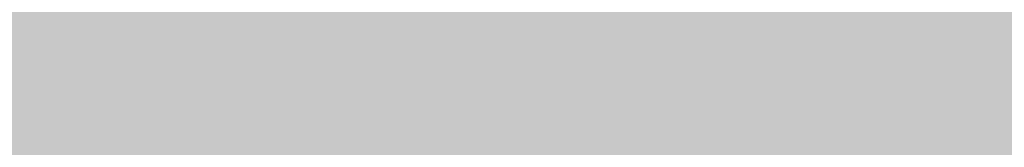
# Model space of a CAD drawing. Units: inches. Extents: x 2083 to 3317, y 1141 to 2115.
# Tile 68 of 256: x 2238.294 to 2242.452, y 1477.116 to 1477.656. Entities that reach past the tile are written whole.
import ezdxf

# ---------------------------------------------------------------- set-up
doc = ezdxf.new("R2010")
doc.units = ezdxf.units.IN
doc.layers.add('A-ANNO-DIMS', color=2, linetype='Continuous', lineweight=18)
doc.layers.add('A-WALL-PATT', color=251, linetype='Continuous', lineweight=13, true_color=0x636466)
doc.styles.get("Standard").update_dxf_attribs({"font": 'arial.ttf'})
doc.dimstyles.new('ISO-25', dxfattribs={"dimtxt": 12, "dimasz": 12, "dimexe": 1.25, "dimexo": 0.625, "dimtad": 1, "dimlunit": 3, "dimtxsty": 'Standard', "dimcen": 2.5, "dimadec": 0, "dimazin": 0, "dimtfac": 1, "dimtmove": 0, "dimatfit": 3, "dimfxl": 1, "dimarcsym": 0})

# ---------------------------------------------------------------- blocks, each defined once
blk = doc.blocks.new('*D30')
at = {"layer": 'A-ANNO-DIMS', "color": 0, "lineweight": -2, "transparency": 16777216}
for p, q in [((2240.0179, 1445.2738), (2240.0179, 1448.0455)), ((2254.3293, 1445.2738), (2254.3293, 1448.0455)), ((2228.0179, 1446.7955), (2216.0179, 1446.7955)), ((2240.0179, 1446.7955), (2254.3293, 1446.7955)), ((2266.3293, 1446.7955), (2413.7649, 1446.7955))]:
    blk.add_line(p, q, dxfattribs=at)
at = {"layer": 'A-ANNO-DIMS', "color": 0, "transparency": 16777216}
for points in [[(2228.0179, 1448.7955), (2228.0179, 1444.7955), (2240.0179, 1446.7955)], [(2266.3293, 1448.7955), (2266.3293, 1444.7955), (2254.3293, 1446.7955)]]:
    blk.add_solid(points, dxfattribs=at)
at = {"layer": 'Defpoints', "color": 0, "transparency": 16777216}
for p in [(2254.3293, 1446.7955), (2240.0179, 1444.6488), (2254.3293, 1444.6488)]:
    blk.add_point(p, dxfattribs=at)
at = {"layer": 'A-ANNO-DIMS', "color": 0, "transparency": 16777216, "insert": (2346.0471, 1453.6252), "char_height": 12, "attachment_point": 5}
blk.add_mtext('WC 1\'-2 1/2" TYP.', dxfattribs=at)
blk = doc.blocks.new('*D31')
at = {"layer": 'A-ANNO-DIMS', "color": 0, "lineweight": -2, "transparency": 16777216}
for p, q in [((2237.8711, 1456.6488), (2237.8711, 1541.9152)), ((2239.3929, 1444.6488), (2236.6211, 1444.6488)), ((2237.8711, 1431.5475), (2237.8711, 1444.6488)), ((2239.3929, 1431.5475), (2236.6211, 1431.5475)), ((2237.8711, 1419.5475), (2237.8711, 1407.5475))]:
    blk.add_line(p, q, dxfattribs=at)
at = {"layer": 'A-ANNO-DIMS', "color": 0, "transparency": 16777216}
for points in [[(2235.8711, 1456.6488), (2239.8711, 1456.6488), (2237.8711, 1444.6488)], [(2235.8711, 1419.5475), (2239.8711, 1419.5475), (2237.8711, 1431.5475)]]:
    blk.add_solid(points, dxfattribs=at)
at = {"layer": 'Defpoints', "color": 0, "transparency": 16777216}
for p in [(2237.8711, 1444.6488), (2240.0179, 1444.6488), (2240.0179, 1431.5475)]:
    blk.add_point(p, dxfattribs=at)
at = {"layer": 'A-ANNO-DIMS', "color": 0, "transparency": 16777216, "insert": (2231.2175, 1505.282), "char_height": 12, "attachment_point": 5, "rotation": 90}
blk.add_mtext('1\'-1" TYP.', dxfattribs=at)
blk = doc.blocks.new('*D62')
at = {"layer": 'A-ANNO-DIMS', "color": 0, "lineweight": -2, "transparency": 16777216}
for p, q in [((2235.9598, 1469.3864), (2235.9598, 1522.3614)), ((2379.9598, 1469.3864), (2379.9598, 1522.3614)), ((2247.9598, 1521.1114), (2367.9598, 1521.1114))]:
    blk.add_line(p, q, dxfattribs=at)
at = {"layer": 'A-ANNO-DIMS', "color": 0, "transparency": 16777216}
for points in [[(2247.9598, 1523.1114), (2247.9598, 1519.1114), (2235.9598, 1521.1114)], [(2367.9598, 1523.1114), (2367.9598, 1519.1114), (2379.9598, 1521.1114)]]:
    blk.add_solid(points, dxfattribs=at)
at = {"layer": 'Defpoints', "color": 0, "transparency": 16777216}
for p in [(2379.9598, 1521.1114), (2235.9598, 1468.7614), (2379.9598, 1468.7614)]:
    blk.add_point(p, dxfattribs=at)
at = {"layer": 'A-ANNO-DIMS', "color": 0, "transparency": 16777216, "insert": (2307.9598, 1527.8632), "char_height": 12, "attachment_point": 5}
blk.add_mtext('12\'-0"', dxfattribs=at)

msp = doc.modelspace()

# ---------------------------------------------------------------- hatches: boundary and pattern name
at = {"layer": 'A-WALL-PATT'}
h = msp.add_hatch(color=256, dxfattribs=at)
h.dxf.hatch_style = 1
h.paths.add_polyline_path([(3126.9598, 2020.7614), (2748.9598, 2020.7614), (2604.9598, 2020.7614), (2226.9598, 2020.7614), (2226.9598, 1702.7614), (2466.9598, 1702.7614), (2466.9598, 1582.7614), (2418.9598, 1582.7614), (2418.9598, 1477.7614), (2226.9598, 1477.7614), (2226.9598, 1263.2614), (2544.9598, 1263.2614), (2544.9598, 1411.7614), (2604.9598, 1411.7614), (2685.9598, 1411.7614), (2685.9598, 1420.7614), (2604.9598, 1420.7614), (2604.9598, 1573.7614), (2604.9598, 1702.7614), (2604.9598, 2011.7614), (2748.9598, 2011.7614), (2748.9598, 1702.7614), (2862.9598, 1702.7614), (2862.9598, 1621.7614), (2871.9598, 1621.7614), (2871.9598, 1702.7614), (2883.9598, 1702.7614), (2883.9598, 1706.9395, -0.026459), (2883.9598, 1711.7614), (2757.9598, 1711.7614), (2757.9598, 1807.7614), (2787.9598, 1807.7614), (2787.9598, 1812.2614), (2757.9598, 1812.2614), (2757.9598, 2011.7614), (2877.9598, 2011.7614), (2877.9598, 1812.2614), (2847.9598, 1812.2614), (2847.9598, 1807.7614), (2889.8357, 1807.7614), (2889.8357, 1812.2614), (2882.4598, 1812.2614), (2882.4598, 2011.7614), (3117.9598, 2011.7614), (3117.9598, 1812.2614), (2937.8357, 1812.2614), (2937.8357, 1807.7614), (2995.7098, 1807.7614), (2995.7098, 1796.1177), (3000.2098, 1796.1177), (3000.2098, 1807.7614), (3117.9598, 1807.7614), (3117.9598, 1711.7614), (3000.2098, 1711.7614), (3000.2098, 1760.1177), (2998.5727, 1760.1177, -0.020711), (2995.7098, 1760.1177), (2995.7098, 1711.7614), (2931.9598, 1711.7614), (2931.9598, 1702.7614), (3126.9598, 1702.7614)])
h.paths.add_polyline_path([(2471.4598, 2011.7614), (2471.4598, 1810.0114), (2462.7169, 1810.0114), (2462.7169, 1805.5114), (2505.9598, 1805.5114), (2505.9598, 1810.0114), (2475.9598, 1810.0114), (2475.9598, 2011.7614), (2595.9598, 2011.7614), (2595.9598, 1810.0114), (2565.9598, 1810.0114), (2565.9598, 1805.5114), (2595.9598, 1805.5114), (2595.9598, 1711.7614), (2235.9598, 1711.7614), (2235.9598, 1805.5114), (2353.7098, 1805.5114), (2353.7098, 1796.0542), (2358.2098, 1796.0542), (2358.2098, 1805.5114), (2414.7169, 1805.5114), (2414.7169, 1810.0114), (2235.9598, 1810.0114), (2235.9598, 2011.7614)], flags=16)
h.paths.add_polyline_path([(2270.2047, 1994.61), (2270.2047, 1970.61), (2246.2047, 1970.61), (2246.2047, 1994.61)], flags=0)
edge = h.paths.add_edge_path(flags=0)
edge.add_ellipse((2332.0274, 1899.7982), major_axis=(-3.043, 3.043), ratio=0.168252, start_angle=-161.3322, end_angle=-156.3071, ccw=False)
edge.add_ellipse((2333.082, 1898.7435), major_axis=(-1.0546, 1.0546), ratio=0.453532, start_angle=-123.371, end_angle=-94.1591)
edge = h.paths.add_edge_path(flags=0)
edge.add_ellipse((2332.0274, 1968.8763), major_axis=(3.043, 3.043), ratio=0.168252, start_angle=18.6678, end_angle=23.6929)
edge.add_spline(control_points=[(2332.9256, 1970.6911), (2332.2268, 1970.3361), (2330.8937, 1969.6589), (2328.4131, 1970.9321), (2327.2039, 1967.7487), (2324.7096, 1969.9556), (2322.5328, 1967.0124), (2320.0128, 1971.2958), (2317.6803, 1968.1578), (2316.0405, 1967.102), (2315.4269, 1966.8096)], knot_values=[0, 0, 0, 0, 2.267059, 4.324559, 6.685584, 8.878641, 11.121502, 14.300359, 17.755284, 19.732645, 19.732645, 19.732645, 19.732645], degree=3, periodic=0)
edge.add_ellipse((2332.0274, 1968.8763), major_axis=(3.043, 3.043), ratio=0.168252, start_angle=18.6678, end_angle=23.6929, ccw=False)
edge.add_ellipse((2333.082, 1969.9309), major_axis=(1.0546, 1.0546), ratio=0.453532, start_angle=56.629, end_angle=85.8409, ccw=False)
edge = h.paths.add_edge_path(flags=0)
edge.add_spline(control_points=[(2296.4283, 1967.9879), (2293.6278, 1965.3363), (2287.7036, 1959.7271), (2299.7439, 1949.9957), (2294.5326, 1935.6685), (2290.5732, 1920.6035), (2293.3941, 1909.9737), (2296.1854, 1904.9665)], knot_values=[0.099185, 0.099185, 0.099185, 0.099185, 0.345301, 0.619822, 0.982653, 1.386093, 1.810555, 1.810555, 1.810555, 1.810555], degree=3, periodic=0)
edge.add_spline(control_points=[(2296.1854, 1904.9665), (2297.3836, 1902.6193), (2298.001, 1901.9493), (2298.553, 1901.4682)], knot_values=[0.006246, 0.006246, 0.006246, 0.006246, 0.055476, 0.055476, 0.055476, 0.055476], degree=3, periodic=0)
edge.add_spline(control_points=[(2298.553, 1901.4682), (2297.2586, 1900.9232), (2295.2253, 1900.2321), (2293.0602, 1900.6142), (2292.1014, 1900.7884), (2292.0896, 1900.7906)], knot_values=[0.312835, 0.312835, 0.312835, 0.312835, 0.40178, 0.474987, 0.475903, 0.475903, 0.475903, 0.475903], degree=3, periodic=0)
edge.add_arc((2292.7936, 1904.6641), 3.937, 215.4209, 259.6982, ccw=False)
edge.add_spline(control_points=[(2289.5853, 1902.3823), (2289.4767, 1902.5351), (2289.3685, 1902.688), (2289.2609, 1902.8412)], knot_values=[0.102872, 0.102872, 0.102872, 0.102872, 0.116896, 0.116896, 0.116896, 0.116896], degree=3, periodic=0)
edge.add_spline(control_points=[(2289.2609, 1902.8412), (2288.6866, 1902.5502), (2287.64, 1902.0199), (2285.8813, 1901.874), (2283.853, 1901.5044), (2281.72, 1899.7105), (2278.467, 1899.4929), (2276.1571, 1901.8832), (2272.259, 1899.8041), (2267.7776, 1901.8432), (2262.2439, 1900.184), (2257.4149, 1901.7821), (2254.3184, 1900.7261), (2253.1783, 1900.3373)], knot_values=[0, 0, 0, 0, 1.907977, 3.477176, 5.261074, 7.972851, 11.680248, 13.717921, 16.939592, 22.789562, 27.502503, 33.595215, 37.145618, 37.145618, 37.145618, 37.145618], degree=3, periodic=0)
edge.add_line((2253.1783, 1900.3373), (2250.2442, 1902.8412))
edge.add_line((2250.2442, 1902.8412), (2250.2442, 1965.8333))
edge.add_line((2250.2442, 1965.8333), (2253.1783, 1968.3371))
edge.add_spline(control_points=[(2253.1783, 1968.3371), (2254.3184, 1967.9483), (2257.4149, 1966.8924), (2262.2439, 1968.4904), (2267.7776, 1966.8313), (2271.5267, 1968.5372), (2273.8759, 1967.8283), (2274.2067, 1967.7276)], knot_values=[0, 0, 0, 0, 0.09018, 0.244935, 0.364644, 0.513233, 0.537855, 0.537855, 0.537855, 0.537855], degree=3, periodic=0)
edge.add_arc((2274.3529, 1963.7933), 3.937, 72.0511, 92.1279, ccw=False)
edge.add_arc((2281.2969, 1985.23), 18.5963, 252.05113, 288.56572)
edge.add_arc((2292.3167, 1956.0289), 12.6461, 71.02679, 113.77822, ccw=False)
edge = h.paths.add_edge_path(flags=0)
edge.add_spline(control_points=[(2274.8994, 1951.8562), (2275.0662, 1951.6166), (2275.2327, 1951.3766), (2275.398, 1951.1359)], knot_values=[1.409916, 1.409916, 1.409916, 1.409916, 1.43159, 1.43159, 1.43159, 1.43159], degree=3, periodic=0)
edge.add_spline(control_points=[(2275.398, 1951.1359), (2275.7921, 1950.5619), (2276.1792, 1949.9838), (2276.5455, 1949.3971)], knot_values=[1.358238, 1.358238, 1.358238, 1.358238, 1.409916, 1.409916, 1.409916, 1.409916], degree=3, periodic=0)
edge.add_line((2276.5455, 1949.3971), (2277.4373, 1947.8622))
edge.add_spline(control_points=[(2277.4373, 1947.8622), (2276.3038, 1945.6731), (2274.6397, 1942.4269), (2274.6316, 1938.0939), (2272.7991, 1930.8515), (2274.3564, 1943.897), (2275.9477, 1947.9234), (2276.5455, 1949.3971)], knot_values=[0.005632, 0.005632, 0.005632, 0.005632, 0.186014, 0.266002, 0.357087, 0.59639, 0.739732, 0.739732, 0.739732, 0.739732], degree=3, periodic=0)
edge.add_spline(control_points=[(2276.5455, 1949.3971), (2276.1792, 1949.9838), (2275.7921, 1950.5619), (2275.398, 1951.1359)], knot_values=[1.358238, 1.358238, 1.358238, 1.358238, 1.409916, 1.409916, 1.409916, 1.409916], degree=3, periodic=0)
edge.add_spline(control_points=[(2275.398, 1951.1359), (2274.9425, 1950.0805), (2274.2078, 1948.0253), (2273.9346, 1944.8515), (2272.4685, 1937.6275), (2273.4662, 1945.6965), (2274.7006, 1951.0595), (2274.8994, 1951.8562)], knot_values=[0.104364, 0.104364, 0.104364, 0.104364, 0.189636, 0.269624, 0.36071, 0.600013, 0.644622, 0.644622, 0.644622, 0.644622], degree=3, periodic=0)
h.paths.add_polyline_path([(2269.1675, 1963.1276, -0.357527), (2268.1706, 1960.9764, -0.092561), (2268.1706, 1939.4363, -0.357527), (2269.1675, 1937.2851, -0.357527), (2267.0163, 1938.282, -0.164785), (2254.6856, 1938.282, -0.357527), (2252.5344, 1937.2851, -0.357527), (2253.5313, 1939.4363, -0.092561), (2253.5313, 1960.9764, -0.357527), (2252.5344, 1963.1276, -0.357527), (2254.6856, 1962.1307, -0.164785), (2267.0163, 1962.1307, -0.357527)], flags=0)
h.paths.add_polyline_path([(2248.8741, 1967.8018), (2248.8741, 1957.0277), (2249.4578, 1957.0277), (2249.4578, 1911.6468), (2248.8741, 1911.6468), (2248.8741, 1900.8727), (2246.5119, 1900.8727, 0.197327), (2244.1497, 1902.4569), (2244.1497, 1966.2176, 0.197327), (2246.5119, 1967.8018)], flags=0)
h.paths.add_polyline_path([(2269.1675, 1931.3893, -0.357527), (2268.1706, 1929.2381, -0.092561), (2268.1706, 1907.6981, -0.357527), (2269.1675, 1905.5469, -0.357527), (2267.0163, 1906.5438, -0.164785), (2254.6856, 1906.5438, -0.357527), (2252.5344, 1905.5469, -0.357527), (2253.5313, 1907.6981, -0.092561), (2253.5313, 1929.2381, -0.357527), (2252.5344, 1931.3893, -0.357527), (2254.6856, 1930.3925, -0.164785), (2267.0163, 1930.3925, -0.357527)], flags=0)
edge = h.paths.add_edge_path(flags=0)
edge.add_spline(control_points=[(2276.1969, 1906.7237), (2276.1681, 1909.0289), (2276.114, 1913.3719), (2270.5984, 1924.925), (2273.9052, 1919.0128), (2275.9217, 1916.2621), (2275.4746, 1912.4021), (2277.2579, 1910.3806), (2276.696, 1908.225), (2276.6462, 1906.813), (2276.6178, 1906.0084)], knot_values=[0, 0, 0, 0, 8.61026, 16.221274, 18.843057, 23.804898, 27.440828, 29.356102, 31.203478, 33.650687, 33.650687, 33.650687, 33.650687], degree=3, periodic=0)
edge.add_spline(control_points=[(2276.6178, 1906.0084), (2276.6233, 1905.6241), (2276.4977, 1904.6287), (2275.4418, 1903.8547), (2274.9373, 1903.0804), (2274.8591, 1902.8412)], knot_values=[0.156488, 0.156488, 0.156488, 0.156488, 0.184398, 0.231376, 0.250598, 0.250598, 0.250598, 0.250598], degree=3, periodic=0)
edge.add_line((2274.8591, 1902.8412), (2276.506, 1902.8412))
edge.add_spline(control_points=[(2276.506, 1902.8412), (2276.7883, 1903.0849), (2277.6651, 1904.1252), (2278.2495, 1904.3407), (2277.6539, 1908.5274), (2278.1557, 1906.2278), (2278.1005, 1905.2859), (2278.8467, 1904.069), (2277.8568, 1903.4149), (2277.8742, 1902.991), (2277.9036, 1902.8412)], knot_values=[0.059574, 0.059574, 0.059574, 0.059574, 0.080753, 0.103741, 0.16972, 0.176036, 0.207137, 0.240474, 0.262341, 0.27366, 0.27366, 0.27366, 0.27366], degree=3, periodic=0)
edge.add_line((2277.9036, 1902.8412), (2280.0298, 1902.8412))
edge.add_spline(control_points=[(2280.0298, 1902.8412), (2279.8882, 1903.0884), (2279.4993, 1903.9816), (2280.1523, 1905.9393), (2278.1036, 1909.6578), (2279.7624, 1907.1853), (2280.3279, 1904.8749), (2280.4851, 1903.4896), (2281.4633, 1903.2494), (2281.7583, 1902.9365), (2281.834, 1902.8412)], knot_values=[0.013856, 0.013856, 0.013856, 0.013856, 0.034874, 0.088867, 0.107879, 0.126738, 0.158714, 0.193757, 0.217487, 0.226722, 0.226722, 0.226722, 0.226722], degree=3, periodic=0)
edge.add_spline(control_points=[(2281.834, 1902.8412), (2281.7875, 1902.8267), (2281.647, 1902.783), (2281.3955, 1902.8595), (2281.0881, 1902.9852), (2280.7207, 1903.0609), (2280.3335, 1903.0257), (2280.1248, 1902.8989), (2280.0298, 1902.8412)], knot_values=[0, 0, 0, 0, 0.14413, 0.435517, 0.749276, 1.153046, 1.548371, 1.878348, 1.878348, 1.878348, 1.878348], degree=3, periodic=0)
edge.add_line((2280.0298, 1902.8412), (2277.9036, 1902.8412))
edge.add_spline(control_points=[(2277.9036, 1902.8412), (2277.8929, 1902.7959), (2277.8654, 1902.6796), (2277.6075, 1902.6875), (2277.2741, 1902.8007), (2276.8379, 1902.6198), (2276.5838, 1902.7893), (2276.506, 1902.8412)], knot_values=[0, 0, 0, 0, 0.127189, 0.326199, 0.628009, 1.24357, 1.515331, 1.515331, 1.515331, 1.515331], degree=3, periodic=0)
edge.add_line((2276.506, 1902.8412), (2274.8591, 1902.8412))
edge.add_spline(control_points=[(2274.8591, 1902.8412), (2274.8144, 1902.8986), (2274.7251, 1903.0134), (2274.4935, 1903.119), (2274.2443, 1902.9605), (2273.9371, 1903.1849), (2273.614, 1902.9831), (2273.4083, 1902.883), (2273.3223, 1902.8412)], knot_values=[0, 0, 0, 0, 0.21843, 0.436957, 0.687977, 0.990379, 1.398396, 1.69185, 1.69185, 1.69185, 1.69185], degree=3, periodic=0)
edge.add_spline(control_points=[(2273.3223, 1902.8412), (2273.6167, 1903.4457), (2274.274, 1904.5383), (2276.0272, 1904.5737), (2276.207, 1906.5836), (2276.1969, 1906.7237)], knot_values=[0.012227, 0.012227, 0.012227, 0.012227, 0.059472, 0.106218, 0.134458, 0.134458, 0.134458, 0.134458], degree=3, periodic=0)
h.paths.add_polyline_path([(2270.7761, 1897.7898), (2270.7761, 1873.7898), (2246.7761, 1873.7898), (2246.7761, 1897.7898)], flags=0)
h.paths.add_polyline_path([(2353.7098, 1760.0051), (2353.7098, 1760.0542), (2358.2098, 1760.0542, -0.033729)], flags=0)
h.paths.add_polyline_path([(2321.8191, 1737.5292), (2341.9953, 1737.5292, -0.414214), (2343.2033, 1736.3212), (2343.2033, 1721.0206, -0.414214), (2341.9953, 1719.8127), (2321.8191, 1719.8127, -0.414214), (2320.6112, 1721.0206), (2320.6112, 1736.3212, -0.414214)], flags=0)
h.paths.add_polyline_path([(2324.235, 1736.3212), (2339.5794, 1736.3212, -0.414214), (2341.9953, 1733.9053), (2341.9953, 1725.4497, -0.414214), (2339.5794, 1723.0338), (2333.6806, 1723.0338), (2333.8453, 1722.0455, -0.870646), (2335.4254, 1721.8259, -0.767327), (2333.9227, 1721.4232), (2331.291, 1721.4232, -0.767327), (2329.7883, 1721.8259, -0.870646), (2331.3684, 1722.0455), (2331.5331, 1723.0338), (2324.235, 1723.0338, -0.414214), (2321.8191, 1725.4497), (2321.8191, 1733.9053, -0.414214)], flags=0)
h.paths.add_polyline_path([(2570.4838, 1928.6154), (2589.6838, 1928.6154), (2590.1688, 1928.6154), (2590.1688, 1904.9934), (2570.4838, 1904.9934)], flags=0)
h.paths.add_polyline_path([(2574.4473, 1927.2638, -1), (2572.8288, 1927.2638, -1)], flags=0)
h.paths.add_polyline_path([(2573.0899, 1926.9409), (2573.925, 1927.776), (2574.1477, 1927.5533), (2573.3126, 1926.7182)], flags=0)
h.paths.add_polyline_path([(2578.7791, 1919.7296, -1), (2571.5917, 1919.7296, -1)], flags=0)
h.paths.add_polyline_path([(2578.3854, 1919.7296, -1), (2571.9854, 1919.7296, -1)], flags=0)
h.paths.add_polyline_path([(2331.5958, 1729.4762, -1), (2333.618, 1729.4762, -1)], flags=0)
h.paths.add_polyline_path([(2578.0342, 1927.2638, -1), (2576.4157, 1927.2638, -1)], flags=0)
h.paths.add_polyline_path([(2576.6889, 1927.5311), (2576.9116, 1927.7538), (2577.7467, 1926.9186), (2577.524, 1926.6959)], flags=0)
h.paths.add_polyline_path([(2578.1391, 1909.8595, -1), (2572.2317, 1909.8595, -1)], flags=0)
h.paths.add_polyline_path([(2577.7454, 1909.8595, -1), (2572.6254, 1909.8595, -1)], flags=0)
h.paths.add_polyline_path([(2583.7977, 1927.2638, -1), (2582.1792, 1927.2638, -1)], flags=0)
h.paths.add_polyline_path([(2582.7186, 1927.7538), (2583.5538, 1926.9186), (2583.3311, 1926.6959), (2582.4959, 1927.5311)], flags=0)
h.paths.add_polyline_path([(2582.4959, 1927.5311), (2582.7186, 1927.7538), (2583.5538, 1926.9186), (2583.3311, 1926.6959)], flags=0)
h.paths.add_polyline_path([(2587.7391, 1920.5296, -1), (2581.8317, 1920.5296, -1)], flags=0)
h.paths.add_polyline_path([(2587.3454, 1920.5296, -1), (2582.2254, 1920.5296, -1)], flags=0)
h.paths.add_polyline_path([(2587.3846, 1927.2638, -1), (2585.7661, 1927.2638, -1)], flags=0)
h.paths.add_polyline_path([(2586.082, 1926.9802), (2586.9172, 1927.8154), (2587.1399, 1927.5927), (2586.3047, 1926.7575)], flags=0)
h.paths.add_polyline_path([(2588.3791, 1910.6595, -1), (2581.1917, 1910.6595, -1)], flags=0)
h.paths.add_polyline_path([(2587.9854, 1910.6595, -1), (2581.5854, 1910.6595, -1)], flags=0)
h.paths.add_polyline_path([(2417.1677, 1729.4779), (2437.3439, 1729.4779, -0.414214), (2438.5519, 1728.2699), (2438.5519, 1712.9693, -0.414214), (2437.3439, 1711.7614), (2417.1677, 1711.7614, -0.414214), (2415.9598, 1712.9693), (2415.9598, 1728.2699, -0.414214)], flags=0)
h.paths.add_polyline_path([(2419.5836, 1728.2699), (2434.928, 1728.2699, -0.414214), (2437.3439, 1725.8541), (2437.3439, 1717.3984, -0.414214), (2434.928, 1714.9825), (2429.0292, 1714.9825), (2429.1939, 1713.9942, -0.870646), (2430.774, 1713.7746, -0.767327), (2429.2713, 1713.372), (2426.6396, 1713.372, -0.767327), (2425.1369, 1713.7746, -0.870646), (2426.717, 1713.9942), (2426.8817, 1714.9825), (2419.5836, 1714.9825, -0.414214), (2417.1677, 1717.3984), (2417.1677, 1725.8541, -0.414214)], flags=0)
h.paths.add_polyline_path([(2419.5836, 1728.2699), (2434.928, 1728.2699, -0.414214), (2437.3439, 1725.8541), (2437.3439, 1717.3984, -0.414214), (2434.928, 1714.9825), (2429.0292, 1714.9825), (2428.3581, 1719.009), (2427.5528, 1719.009), (2426.8817, 1714.9825), (2419.5836, 1714.9825, -0.414214), (2417.1677, 1717.3984), (2417.1677, 1725.8541, -0.414214)], flags=0)
h.paths.add_polyline_path([(2426.9444, 1721.4249, -1), (2428.9666, 1721.4249, -1)], flags=0)
h.paths.add_polyline_path([(2475.9598, 1702.7614), (2595.9598, 1702.7614), (2595.9598, 1582.7614), (2475.9598, 1582.7614)], flags=16)
h.paths.add_polyline_path([(2427.9598, 1573.7614), (2595.9598, 1573.7614), (2595.9598, 1468.7614), (2595.9598, 1420.7614), (2384.4598, 1420.7614), (2384.4598, 1468.7614), (2427.9598, 1468.7614)], flags=16)
h.paths.add_polyline_path([(2379.9598, 1468.7614), (2379.9598, 1420.7614), (2235.9598, 1420.7614), (2235.9598, 1468.7614)], flags=16)
h.paths.add_polyline_path([(2317.816, 1466.6958), (2337.9922, 1466.6958, -0.414214), (2339.2002, 1465.4878), (2339.2002, 1450.1872, -0.414214), (2337.9922, 1448.9792), (2317.816, 1448.9792, -0.414214), (2316.6081, 1450.1872), (2316.6081, 1465.4878, -0.414214)], flags=0)
h.paths.add_polyline_path([(2320.2319, 1465.4878), (2335.5763, 1465.4878, -0.414214), (2337.9922, 1463.0719), (2337.9922, 1454.6163, -0.414214), (2335.5763, 1452.2004), (2329.6775, 1452.2004), (2329.8422, 1451.212, -0.870646), (2331.4223, 1450.9925, -0.767327), (2329.9196, 1450.5898), (2327.2879, 1450.5898, -0.767327), (2325.7852, 1450.9925, -0.870646), (2327.3653, 1451.212), (2327.53, 1452.2004), (2320.2319, 1452.2004, -0.414214), (2317.816, 1454.6163), (2317.816, 1463.0719, -0.414214)], flags=0)
h.paths.add_polyline_path([(2320.2319, 1465.4878), (2335.5763, 1465.4878, -0.414214), (2337.9922, 1463.0719), (2337.9922, 1454.6163, -0.414214), (2335.5763, 1452.2004), (2329.6775, 1452.2004), (2329.0064, 1456.2269), (2328.2011, 1456.2269), (2327.53, 1452.2004), (2320.2319, 1452.2004, -0.414214), (2317.816, 1454.6163), (2317.816, 1463.0719, -0.414214)], flags=0)
h.paths.add_polyline_path([(2327.5926, 1458.6428, -1), (2329.6148, 1458.6428, -1)], flags=0)
h.paths.add_polyline_path([(2244.4117, 1433.3405), (2241.9209, 1433.3405, -0.414214), (2240.0179, 1435.2435), (2240.0179, 1440.9528, -0.414211), (2241.9209, 1442.8559), (2244.4117, 1442.8559, -1.976472)], flags=0)
h.paths.add_polyline_path([(2245.3569, 1434.3975, -0.414214), (2245.3569, 1441.7988, -2.144098)], flags=0)
h.paths.add_polyline_path([(2535.9598, 1416.2614), (2535.9598, 1272.2614), (2235.9598, 1272.2614), (2235.9598, 1416.2614)], flags=16)
h.paths.add_polyline_path([(2260.1196, 1384.2928), (2260.1196, 1362.0386), (2237.8654, 1362.0386), (2237.8654, 1384.2928)], flags=0)
edge = h.paths.add_edge_path(flags=0)
edge.add_line((2318.2518, 1362.0933), (2318.1458, 1362.001))
edge.add_ellipse((2317.4451, 1360.431), major_axis=(2.8216, 2.8216), ratio=0.168252, start_angle=18.6678, end_angle=20.9481, ccw=False)
edge.add_ellipse((2318.423, 1361.409), major_axis=(0.9779, 0.9779), ratio=0.453532, start_angle=56.629, end_angle=70.2262, ccw=False)
edge = h.paths.add_edge_path(flags=0)
edge.add_line((2319.1074, 1295.5711), (2319.015, 1295.6771))
edge.add_ellipse((2317.4451, 1296.3778), major_axis=(-2.8216, 2.8216), ratio=0.168252, start_angle=-161.3322, end_angle=-159.0519, ccw=False)
edge.add_ellipse((2318.423, 1295.3999), major_axis=(-0.9779, 0.9779), ratio=0.453532, start_angle=-123.371, end_angle=-109.7738)
edge = h.paths.add_edge_path(flags=0)
edge.add_spline(control_points=[(2284.2103, 1301.1702), (2284.5807, 1300.4447), (2284.8912, 1299.892), (2285.1596, 1299.461)], knot_values=[0.039066, 0.039066, 0.039066, 0.039066, 0.055476, 0.055476, 0.055476, 0.055476], degree=3, periodic=0)
edge.add_line((2285.1596, 1299.461), (2284.2103, 1301.1702))
edge = h.paths.add_edge_path(flags=0)
edge.add_line((2280.4125, 1297.298), (2283.37, 1297.0361))
edge.add_line((2283.37, 1297.0361), (2286.4057, 1297.9263))
edge.add_spline(control_points=[(2286.4057, 1297.9263), (2285.3055, 1297.4631), (2284.3448, 1297.1292), (2283.37, 1297.0361)], knot_values=[0.394369, 0.394369, 0.394369, 0.394369, 0.475903, 0.475903, 0.475903, 0.475903], degree=3, periodic=0)
edge.add_spline(control_points=[(2283.37, 1297.0361), (2283.2814, 1297.0277), (2282.3163, 1296.9573), (2281.3125, 1297.1345), (2280.4234, 1297.296), (2280.4125, 1297.298)], knot_values=[0.312835, 0.312835, 0.312835, 0.312835, 0.320246, 0.393453, 0.394369, 0.394369, 0.394369, 0.394369], degree=3, periodic=0)
edge = h.paths.add_edge_path(flags=0)
edge.add_line((2284.4356, 1359.6073), (2280.4463, 1355.328))
edge.add_line((2280.4463, 1355.328), (2279.58, 1351.0178))
edge.add_line((2279.58, 1351.0178), (2282.413, 1346.5804))
edge.add_spline(control_points=[(2282.413, 1346.5804), (2283.1533, 1345.5892), (2284.2529, 1344.0289), (2284.801, 1342.3872), (2284.9352, 1341.8055)], knot_values=[1.240098, 1.240098, 1.240098, 1.240098, 1.332892, 1.382712, 1.382712, 1.382712, 1.382712], degree=3, periodic=0)
edge.add_spline(control_points=[(2284.9352, 1341.8055), (2285.3191, 1340.1406), (2285.233, 1338.4092), (2284.9099, 1336.6541)], knot_values=[1.097484, 1.097484, 1.097484, 1.097484, 1.240098, 1.240098, 1.240098, 1.240098], degree=3, periodic=0)
edge.add_spline(control_points=[(2284.9099, 1336.6541), (2284.5868, 1334.899), (2284.0267, 1333.1203), (2283.4626, 1331.3606)], knot_values=[0.95487, 0.95487, 0.95487, 0.95487, 1.097484, 1.097484, 1.097484, 1.097484], degree=3, periodic=0)
edge.add_line((2283.4626, 1331.3606), (2281.8904, 1326.1534))
edge.add_line((2281.8904, 1326.1534), (2280.7563, 1321.0561))
edge.add_line((2280.7563, 1321.0561), (2280.2992, 1316.002))
edge.add_line((2280.2992, 1316.002), (2280.7159, 1310.9501))
edge.add_line((2280.7159, 1310.9501), (2282.0281, 1305.9721))
edge.add_line((2282.0281, 1305.9721), (2284.2103, 1301.1702))
edge.add_spline(control_points=[(2284.2103, 1301.1702), (2283.3407, 1302.7302), (2282.6119, 1304.3365), (2282.0281, 1305.9721)], knot_values=[0.099185, 0.099185, 0.099185, 0.099185, 0.241799, 0.241799, 0.241799, 0.241799], degree=3, periodic=0)
edge.add_spline(control_points=[(2282.0281, 1305.9721), (2281.4443, 1307.6078), (2281.0055, 1309.2728), (2280.7159, 1310.9501)], knot_values=[0.241799, 0.241799, 0.241799, 0.241799, 0.384413, 0.384413, 0.384413, 0.384413], degree=3, periodic=0)
edge.add_spline(control_points=[(2280.7159, 1310.9501), (2280.4332, 1312.5876), (2280.2894, 1314.277), (2280.2989, 1315.962), (2280.2992, 1316.002)], knot_values=[0.384413, 0.384413, 0.384413, 0.384413, 0.523647, 0.527028, 0.527028, 0.527028, 0.527028], degree=3, periodic=0)
edge.add_spline(control_points=[(2280.2992, 1316.002), (2280.3123, 1317.687), (2280.4779, 1319.3679), (2280.7563, 1321.0561)], knot_values=[0.527028, 0.527028, 0.527028, 0.527028, 0.669642, 0.669642, 0.669642, 0.669642], degree=3, periodic=0)
edge.add_spline(control_points=[(2280.7563, 1321.0561), (2281.0346, 1322.7443), (2281.4259, 1324.4396), (2281.8904, 1326.1534)], knot_values=[0.669642, 0.669642, 0.669642, 0.669642, 0.812256, 0.812256, 0.812256, 0.812256], degree=3, periodic=0)
edge.add_spline(control_points=[(2281.8904, 1326.1534), (2282.2644, 1327.5333), (2282.7879, 1329.2618), (2283.3528, 1331.0178), (2283.4626, 1331.3606)], knot_values=[0.812256, 0.812256, 0.812256, 0.812256, 0.927087, 0.95487, 0.95487, 0.95487, 0.95487], degree=3, periodic=0)
edge.add_line((2283.4626, 1331.3606), (2284.9099, 1336.6541))
edge.add_line((2284.9099, 1336.6541), (2284.9352, 1341.8055))
edge.add_line((2284.9352, 1341.8055), (2282.413, 1346.5804))
edge.add_spline(control_points=[(2282.413, 1346.5804), (2281.2751, 1348.1038), (2280.0784, 1349.5703), (2279.58, 1351.0178)], knot_values=[1.382712, 1.382712, 1.382712, 1.382712, 1.525326, 1.525326, 1.525326, 1.525326], degree=3, periodic=0)
edge.add_spline(control_points=[(2279.58, 1351.0178), (2279.4433, 1351.4147), (2279.1363, 1352.8569), (2279.7352, 1354.2904), (2280.4463, 1355.328)], knot_values=[1.525326, 1.525326, 1.525326, 1.525326, 1.564439, 1.667941, 1.667941, 1.667941, 1.667941], degree=3, periodic=0)
edge.add_spline(control_points=[(2280.4463, 1355.328), (2281.4261, 1356.7578), (2282.9308, 1358.1826), (2284.4356, 1359.6073)], knot_values=[1.667941, 1.667941, 1.667941, 1.667941, 1.810555, 1.810555, 1.810555, 1.810555], degree=3, periodic=0)
edge.add_arc((2280.6231, 1348.5182), 11.7262, 71.02679, 113.77822)
edge.add_arc((2270.4049, 1375.5952), 17.2436, 252.05113, 288.56572, ccw=False)
edge.add_arc((2263.966, 1355.7178), 3.6506, 72.0511, 92.1279)
edge.add_arc((2263.966, 1355.7178), 3.6506, 92.1279, 177.9851)
edge.add_spline(control_points=[(2260.3176, 1355.8462), (2260.2604, 1354.2207), (2260.5513, 1350.1865), (2262.9993, 1346.7663), (2264.4727, 1344.649)], knot_values=[1.43159, 1.43159, 1.43159, 1.43159, 1.564144, 1.770695, 1.770695, 1.770695, 1.770695], degree=3, periodic=0)
edge.add_line((2264.4727, 1344.649), (2264.9356, 1343.9825))
edge.add_spline(control_points=[(2263.801, 1340.2481), (2263.8432, 1340.5141), (2264.0672, 1341.7565), (2264.5127, 1343.0025), (2264.935, 1343.9811)], knot_values=[0.53657, 0.53657, 0.53657, 0.53657, 0.559349, 0.644622, 0.644622, 0.644622, 0.644622], degree=3, periodic=0)
edge.add_spline(control_points=[(2264.935, 1343.9811), (2265.1178, 1343.715), (2265.2989, 1343.4479), (2265.4768, 1343.1794)], knot_values=[1.384077, 1.384077, 1.384077, 1.384077, 1.409916, 1.409916, 1.409916, 1.409916], degree=3, periodic=0)
edge.add_spline(control_points=[(2265.4768, 1343.1794), (2265.6546, 1342.9108), (2265.8293, 1342.6408), (2265.9991, 1342.3688)], knot_values=[1.358238, 1.358238, 1.358238, 1.358238, 1.384077, 1.384077, 1.384077, 1.384077], degree=3, periodic=0)
edge.add_line((2265.9991, 1342.3688), (2266.826, 1340.9455))
edge.add_spline(control_points=[(2266.826, 1340.9455), (2268.8944, 1337.0897), (2271.3982, 1325.843), (2270.5162, 1310.5686), (2275.9194, 1301.8606), (2277.7895, 1299.1994)], knot_values=[0.116896, 0.116896, 0.116896, 0.116896, 0.472987, 1.050969, 1.313793, 1.313793, 1.313793, 1.313793], degree=3, periodic=0)
edge.add_spline(control_points=[(2277.7895, 1299.1994), (2277.8394, 1299.1285), (2277.8894, 1299.0575), (2277.9396, 1298.9866)], knot_values=[0.109884, 0.109884, 0.109884, 0.109884, 0.116896, 0.116896, 0.116896, 0.116896], degree=3, periodic=0)
edge.add_line((2277.9396, 1298.9866), (2277.7888, 1299.1991))
edge.add_spline(control_points=[(2277.7888, 1299.1991), (2277.2566, 1298.9294), (2276.2864, 1298.4379), (2275.0394, 1298.3344), (2274.3833, 1298.2389), (2274.2153, 1298.2093)], knot_values=[33.12187, 33.12187, 33.12187, 33.12187, 35.029056, 36.598255, 37.144827, 37.144827, 37.144827, 37.144827], degree=3, periodic=0)
edge.add_line((2274.2153, 1298.2093), (2273.0731, 1297.893))
edge.add_spline(control_points=[(2273.0731, 1297.893), (2272.3229, 1297.5798), (2271.0392, 1296.5105), (2269.2484, 1296.2261), (2268.4231, 1296.3747)], knot_values=[26.532584, 26.532584, 26.532584, 26.532584, 29.198919, 31.839101, 31.839101, 31.839101, 31.839101], degree=3, periodic=0)
edge.add_line((2268.4231, 1296.3747), (2263.8785, 1297.4575))
edge.add_spline(control_points=[(2263.8785, 1297.4575), (2263.5561, 1297.3594), (2261.8603, 1296.8387), (2260.2388, 1297.2824), (2258.9335, 1297.5165)], knot_values=[15.919551, 15.919551, 15.919551, 15.919551, 16.939592, 21.226067, 21.226067, 21.226067, 21.226067], degree=3, periodic=0)
edge.add_line((2258.9335, 1297.5165), (2254.0552, 1297.329))
edge.add_spline(control_points=[(2254.0552, 1297.329), (2253.7555, 1297.2958), (2252.1137, 1297.1652), (2250.4619, 1297.5442), (2249.1297, 1297.6679)], knot_values=[5.306517, 5.306517, 5.306517, 5.306517, 6.276435, 10.613034, 10.613034, 10.613034, 10.613034], degree=3, periodic=0)
edge.add_line((2249.1297, 1297.6679), (2244.3316, 1296.8778))
edge.add_line((2244.3316, 1296.8778), (2241.611, 1299.1994))
edge.add_line((2241.611, 1299.1994), (2241.611, 1357.6094))
edge.add_line((2241.611, 1357.6094), (2244.3316, 1359.9311))
edge.add_line((2244.3316, 1359.9311), (2252.7288, 1359.5427))
edge.add_spline(control_points=[(2252.7288, 1359.5427), (2252.8709, 1359.5464), (2253.3057, 1359.5482), (2253.7398, 1359.5143), (2254.0317, 1359.4824)], knot_values=[0.233291, 0.233291, 0.233291, 0.233291, 0.244935, 0.268927, 0.268927, 0.268927, 0.268927], degree=3, periodic=0)
edge.add_line((2254.0317, 1359.4824), (2259.5872, 1359.4164))
edge.add_spline(control_points=[(2259.5872, 1359.4164), (2260.6771, 1359.6285), (2262.0732, 1359.897), (2263.5237, 1359.4593), (2263.8304, 1359.366)], knot_values=[0.422516, 0.422516, 0.422516, 0.422516, 0.513233, 0.537855, 0.537855, 0.537855, 0.537855], degree=3, periodic=0)
edge.add_arc((2263.966, 1355.7178), 3.6506, 72.0511, 92.1279, ccw=False)
edge.add_arc((2270.4049, 1375.5952), 17.2436, 252.05113, 288.56572)
edge.add_arc((2280.6231, 1348.5182), 11.7262, 71.02679, 113.77822, ccw=False)
h.paths.add_polyline_path([(2240.3405, 1359.4347), (2240.3405, 1349.4444), (2240.8818, 1349.4444), (2240.8818, 1307.3645), (2240.3405, 1307.3645), (2240.3405, 1297.3741), (2238.1502, 1297.3741, 0.197327), (2235.9598, 1298.8431), (2235.9598, 1357.9657, 0.197327), (2238.1502, 1359.4347)], flags=0)
h.paths.add_polyline_path([(2259.1578, 1355.1005, -0.357527), (2258.2334, 1353.1058, -0.092561), (2258.2334, 1333.1326, -0.357527), (2259.1578, 1331.1379, -0.357527), (2257.1631, 1332.0622, -0.164785), (2245.7293, 1332.0622, -0.357527), (2243.7346, 1331.1379, -0.357527), (2244.6589, 1333.1326, -0.092561), (2244.6589, 1353.1058, -0.357527), (2243.7346, 1355.1005, -0.357527), (2245.7293, 1354.1761, -0.164785), (2257.1631, 1354.1761, -0.357527)], flags=0)
edge = h.paths.add_edge_path(flags=0)
edge.add_line((2265.9991, 1342.3688), (2266.826, 1340.9455))
edge.add_line((2266.826, 1340.9455), (2265.3076, 1337.8141))
edge.add_line((2265.3076, 1337.8141), (2264.3582, 1334.6529))
edge.add_line((2264.3582, 1334.6529), (2264.262, 1333.7997))
edge.add_spline(control_points=[(2264.262, 1333.7997), (2264.2084, 1333.1871), (2264.1621, 1332.3655), (2264.0071, 1331.4139), (2263.969, 1331.2018)], knot_values=[0.464444, 0.464444, 0.464444, 0.464444, 0.516691, 0.531608, 0.531608, 0.531608, 0.531608], degree=3, periodic=0)
edge.add_spline(control_points=[(2263.969, 1331.2018), (2263.7745, 1330.1189), (2263.4244, 1328.7908), (2263.2574, 1328.5307), (2263.234, 1328.5146)], knot_values=[0.372682, 0.372682, 0.372682, 0.372682, 0.44885, 0.464444, 0.464444, 0.464444, 0.464444], degree=3, periodic=0)
edge.add_spline(control_points=[(2263.234, 1328.5146), (2263.0964, 1328.4202), (2263.1312, 1329.3015), (2263.275, 1330.6157)], knot_values=[0.280919, 0.280919, 0.280919, 0.280919, 0.372682, 0.372682, 0.372682, 0.372682], degree=3, periodic=0)
edge.add_spline(control_points=[(2263.275, 1330.6157), (2263.4187, 1331.93), (2263.6715, 1333.6773), (2263.9699, 1335.315)], knot_values=[0.189157, 0.189157, 0.189157, 0.189157, 0.280919, 0.280919, 0.280919, 0.280919], degree=3, periodic=0)
edge.add_spline(control_points=[(2263.9699, 1335.315), (2264.1005, 1336.0322), (2264.4188, 1337.6219), (2264.7548, 1338.8644), (2264.9474, 1339.4911)], knot_values=[0.097394, 0.097394, 0.097394, 0.097394, 0.137578, 0.189157, 0.189157, 0.189157, 0.189157], degree=3, periodic=0)
edge.add_spline(control_points=[(2264.9474, 1339.4911), (2265.29, 1340.6061), (2265.6442, 1341.494), (2265.9991, 1342.3688)], knot_values=[0.005632, 0.005632, 0.005632, 0.005632, 0.097394, 0.097394, 0.097394, 0.097394], degree=3, periodic=0)
h.paths.add_polyline_path([(2259.1578, 1325.671, -0.357527), (2258.2334, 1323.6763, -0.092561), (2258.2334, 1303.7031, -0.357527), (2259.1578, 1301.7084, -0.357527), (2257.1631, 1302.6327, -0.164785), (2245.7293, 1302.6327, -0.357527), (2243.7346, 1301.7084, -0.357527), (2244.6589, 1303.7031, -0.092561), (2244.6589, 1323.6763, -0.357527), (2243.7346, 1325.671, -0.357527), (2245.7293, 1324.7466, -0.164785), (2257.1631, 1324.7466, -0.357527)], flags=0)
edge = h.paths.add_edge_path(flags=0)
edge.add_spline(control_points=[(2261.7089, 1317.3114), (2261.6795, 1317.4176), (2261.7619, 1317.3885), (2262.4907, 1316.0899), (2262.9622, 1315.3009)], knot_values=[14.955861, 14.955861, 14.955861, 14.955861, 16.221274, 18.694826, 18.694826, 18.694826, 18.694826], degree=3, periodic=0)
edge.add_spline(control_points=[(2262.9622, 1315.3009), (2262.9904, 1315.2536), (2263.7021, 1314.0674), (2264.349, 1313.1272), (2264.7301, 1312.1642)], knot_values=[18.694826, 18.694826, 18.694826, 18.694826, 18.843057, 22.433791, 22.433791, 22.433791, 22.433791], degree=3, periodic=0)
edge.add_spline(control_points=[(2264.7301, 1312.1642), (2264.8756, 1311.7964), (2265.1769, 1310.7698), (2265.1431, 1309.5593), (2265.2477, 1308.8242)], knot_values=[22.433791, 22.433791, 22.433791, 22.433791, 23.804898, 26.172756, 26.172756, 26.172756, 26.172756], degree=3, periodic=0)
edge.add_line((2265.2477, 1308.8242), (2265.8508, 1307.1719))
edge.add_spline(control_points=[(2265.8508, 1307.1719), (2266.065, 1306.8217), (2266.3844, 1306.3322), (2266.4244, 1305.7805), (2266.4204, 1305.6112)], knot_values=[28.062562, 28.062562, 28.062562, 28.062562, 29.356102, 29.911721, 29.911721, 29.911721, 29.911721], degree=3, periodic=0)
edge.add_spline(control_points=[(2266.4204, 1305.6112), (2266.4161, 1305.4326), (2266.394, 1305.25), (2266.3648, 1305.0659)], knot_values=[29.911721, 29.911721, 29.911721, 29.911721, 30.497837, 30.497837, 30.497837, 30.497837], degree=3, periodic=0)
edge.add_line((2266.3648, 1305.0659), (2266.0662, 1302.1363))
edge.add_spline(control_points=[(2266.0662, 1302.1363), (2266.0712, 1301.78), (2265.9981, 1301.2), (2265.6633, 1300.759), (2265.5089, 1300.5859)], knot_values=[0.156488, 0.156488, 0.156488, 0.156488, 0.184398, 0.203543, 0.203543, 0.203543, 0.203543], degree=3, periodic=0)
edge.add_line((2265.5089, 1300.5859), (2264.4353, 1299.1994))
edge.add_line((2264.4353, 1299.1994), (2265.9624, 1299.1994))
edge.add_line((2265.9624, 1299.1994), (2267.336, 1301.1753))
edge.add_line((2267.336, 1301.1753), (2267.3117, 1301.9862))
edge.add_spline(control_points=[(2267.3117, 1301.9862), (2267.2611, 1302.8624), (2267.1602, 1303.7371), (2267.2715, 1303.3259)], knot_values=[0.126229, 0.126229, 0.126229, 0.126229, 0.166617, 0.166617, 0.166617, 0.166617], degree=3, periodic=0)
edge.add_spline(control_points=[(2267.2715, 1303.3259), (2267.28, 1303.2943), (2267.3098, 1303.1754), (2267.3735, 1302.8836), (2267.4061, 1302.6828), (2267.4179, 1302.601)], knot_values=[0.166617, 0.166617, 0.166617, 0.166617, 0.16972, 0.176036, 0.180765, 0.180765, 0.180765, 0.180765], degree=3, periodic=0)
edge.add_spline(control_points=[(2267.7439, 1300.9875), (2267.6876, 1301.1509), (2267.4805, 1301.6567), (2267.4838, 1302.1448), (2267.4179, 1302.601)], knot_values=[0.180765, 0.180765, 0.180765, 0.180765, 0.193767, 0.220139, 0.220139, 0.220139, 0.220139], degree=3, periodic=0)
edge.add_line((2267.4179, 1302.601), (2267.7439, 1300.9875))
edge.add_spline(control_points=[(2267.7439, 1300.9875), (2267.832, 1300.7319), (2267.932, 1300.3099), (2267.5548, 1299.9745), (2267.4294, 1299.8292)], knot_values=[0.220139, 0.220139, 0.220139, 0.220139, 0.240474, 0.25489, 0.25489, 0.25489, 0.25489], degree=3, periodic=0)
edge.add_line((2267.4294, 1299.8292), (2267.2584, 1299.1994))
edge.add_line((2267.2584, 1299.1994), (2269.23, 1299.1994))
edge.add_spline(control_points=[(2269.23, 1299.1994), (2269.0987, 1299.4287), (2268.8428, 1300.0163), (2269.0116, 1300.9159), (2268.9468, 1301.6607)], knot_values=[0.013856, 0.013856, 0.013856, 0.013856, 0.034874, 0.067073, 0.067073, 0.067073, 0.067073], degree=3, periodic=0)
edge.add_line((2268.9468, 1301.6607), (2268.4316, 1303.6031))
edge.add_spline(control_points=[(2268.4316, 1303.6031), (2268.1756, 1304.1924), (2267.5962, 1305.2513), (2268.0407, 1304.6232), (2268.2514, 1304.2824)], knot_values=[0.090155, 0.090155, 0.090155, 0.090155, 0.107879, 0.120289, 0.120289, 0.120289, 0.120289], degree=3, periodic=0)
edge.add_spline(control_points=[(2268.2514, 1304.2824), (2268.3609, 1304.1053), (2269.0578, 1302.918), (2269.3827, 1301.5904), (2269.5214, 1300.7759), (2269.5752, 1300.5558)], knot_values=[0.120289, 0.120289, 0.120289, 0.120289, 0.126738, 0.158714, 0.173506, 0.173506, 0.173506, 0.173506], degree=3, periodic=0)
edge.add_line((2269.5752, 1300.5558), (2270.6858, 1299.4213))
edge.add_spline(control_points=[(2270.6858, 1299.4213), (2270.7672, 1299.3573), (2270.8379, 1299.2814), (2270.9029, 1299.1994)], knot_values=[0.21816, 0.21816, 0.21816, 0.21816, 0.226722, 0.226722, 0.226722, 0.226722], degree=3, periodic=0)
edge.add_line((2270.9372, 1299.1929), (2270.9029, 1299.1994))
edge.add_spline(control_points=[(2270.9029, 1299.1994), (2270.8598, 1299.186), (2270.7295, 1299.1455), (2270.4963, 1299.2164), (2270.2717, 1299.3083), (2270.121, 1299.348), (2270.0633, 1299.3596)], knot_values=[0.939174, 0.939174, 0.939174, 0.939174, 1.083304, 1.374691, 1.68845, 1.878348, 1.878348, 1.878348, 1.878348], degree=3, periodic=0)
edge.add_line((2270.0633, 1299.3596), (2269.23, 1299.1994))
edge.add_line((2269.23, 1299.1994), (2267.2584, 1299.1994))
edge.add_spline(control_points=[(2267.2584, 1299.1994), (2267.2484, 1299.1574), (2267.223, 1299.0497), (2266.9838, 1299.0569), (2266.8092, 1299.1162), (2266.6769, 1299.1091), (2266.6365, 1299.1048)], knot_values=[0.757665, 0.757665, 0.757665, 0.757665, 0.884854, 1.083864, 1.385675, 1.515331, 1.515331, 1.515331, 1.515331], degree=3, periodic=0)
edge.add_spline(control_points=[(2266.6365, 1299.1048), (2266.4852, 1299.0888), (2266.2358, 1299.0171), (2266.0346, 1299.1513), (2265.9624, 1299.1994)], knot_values=[0, 0, 0, 0, 0.485905, 0.757665, 0.757665, 0.757665, 0.757665], degree=3, periodic=0)
edge.add_line((2265.9624, 1299.1994), (2264.4353, 1299.1994))
edge.add_line((2264.4353, 1299.1994), (2263.8584, 1299.3671))
edge.add_spline(control_points=[(2263.8584, 1299.3671), (2263.8189, 1299.3709), (2263.7795, 1299.3857), (2263.7401, 1299.4015)], knot_values=[0.845925, 0.845925, 0.845925, 0.845925, 0.978627, 0.978627, 0.978627, 0.978627], degree=3, periodic=0)
edge.add_line((2263.7218, 1299.3964), (2263.0103, 1299.1994))
edge.add_spline(control_points=[(2263.0103, 1299.1994), (2263.2458, 1299.6829), (2263.506, 1300.1281), (2263.8735, 1300.408)], knot_values=[0.012227, 0.012227, 0.012227, 0.012227, 0.052971, 0.052971, 0.052971, 0.052971], degree=3, periodic=0)
edge.add_spline(control_points=[(2263.8735, 1300.408), (2263.9321, 1300.4527), (2264.0842, 1300.553), (2264.2552, 1300.6242), (2264.3597, 1300.6647)], knot_values=[0.052971, 0.052971, 0.052971, 0.052971, 0.059472, 0.069086, 0.069086, 0.069086, 0.069086], degree=3, periodic=0)
edge.add_line((2264.3597, 1300.6647), (2265.1419, 1301.0778))
edge.add_line((2265.1419, 1301.0778), (2265.6758, 1302.7996))
edge.add_line((2265.6758, 1302.7996), (2265.5407, 1305.7041))
edge.add_line((2265.5407, 1305.7041), (2264.8031, 1309.3277))
edge.add_line((2264.8031, 1309.3277), (2263.0405, 1314.0918))
edge.add_spline(control_points=[(2263.0405, 1314.0918), (2262.3836, 1315.6714), (2261.796, 1316.9977), (2261.7089, 1317.3114)], knot_values=[11.216896, 11.216896, 11.216896, 11.216896, 14.955861, 14.955861, 14.955861, 14.955861], degree=3, periodic=0)
h.paths.add_polyline_path([(2871.9598, 1416.2614), (2895.91, 1416.2614), (2895.91, 1420.7614), (2871.9598, 1420.7614), (2871.9598, 1501.7614), (2862.9598, 1501.7614), (2862.9598, 1420.7614), (2805.9598, 1420.7614), (2805.9598, 1411.7614), (2862.9598, 1411.7614), (2862.9598, 1263.2614), (3126.9598, 1263.2614), (3126.9598, 1411.7614), (3126.9598, 1486.7614), (2943.9598, 1486.7614), (2943.9598, 1477.7614), (2967.8603, 1477.7614), (2967.8603, 1420.7614), (2943.91, 1420.7614), (2943.91, 1416.2614), (3117.9598, 1416.2614), (3117.9598, 1420.7614), (2972.3603, 1420.7614), (2972.3603, 1477.7614), (3117.9598, 1477.7614), (3117.9598, 1420.7614), (3117.9598, 1272.2614), (2871.9598, 1272.2614)], flags=0)
h.paths.add_polyline_path([(2457.1256, 1485.9425), (2527.6027, 1485.9425), (2527.6027, 1537.6357), (2457.1256, 1537.6357)], flags=8)
h.paths.add_polyline_path([(2481.0051, 1609.9818), (2590.7658, 1609.9818), (2590.7658, 1682.0034), (2481.0051, 1682.0034)], flags=8)
h.paths.add_polyline_path([(2483.085, 1729.1268), (2553.562, 1729.1268), (2553.562, 1780.82), (2483.085, 1780.82)], flags=8)

# ---------------------------------------------------------------- dimensions: what is measured, and where the dimension line sits
at = {"layer": 'A-ANNO-DIMS'}
dim = msp.add_linear_dim(base=(2237.8711, 1444.6488), p1=(2240.0179, 1431.5475), p2=(2240.0179, 1444.6488), angle=90, text='<> TYP.', dimstyle='ISO-25', override={"dimdec": 1, "dimlfac": 1, "dimrnd": 0, "dimzin": 1, "dimdsep": 46, "dimlunit": 4, "dimfrac": 2}, dxfattribs=at)
dim.commit()
dim.dimension.update_dxf_attribs({"geometry": '*D31', "text_midpoint": (2231.2175, 1505.282)})
dim = msp.add_linear_dim(base=(2379.9598, 1521.1114), p1=(2235.9598, 1468.7614), p2=(2379.9598, 1468.7614), dimstyle='ISO-25', override={"dimdec": 1, "dimlfac": 1, "dimrnd": 0, "dimzin": 1, "dimdsep": 46, "dimlunit": 4, "dimfrac": 2}, dxfattribs=at)
dim.commit()
dim.dimension.update_dxf_attribs({"geometry": '*D62', "text_midpoint": (2307.9598, 1527.8632)})
dim = msp.add_linear_dim(base=(2254.3293, 1446.7955), p1=(2240.0179, 1444.6488), p2=(2254.3293, 1444.6488), text='WC <> TYP.', dimstyle='ISO-25', override={"dimdec": 1, "dimlfac": 1, "dimrnd": 0, "dimzin": 1, "dimdsep": 46, "dimlunit": 4, "dimfrac": 2}, dxfattribs=at)
dim.commit()
dim.dimension.update_dxf_attribs({"geometry": '*D30', "text_midpoint": (2346.0471, 1453.6252)})

doc.saveas('drawing.dxf')
